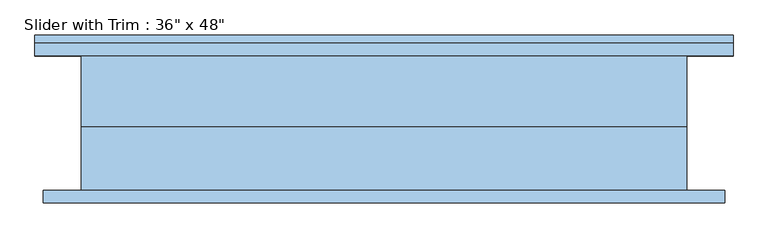
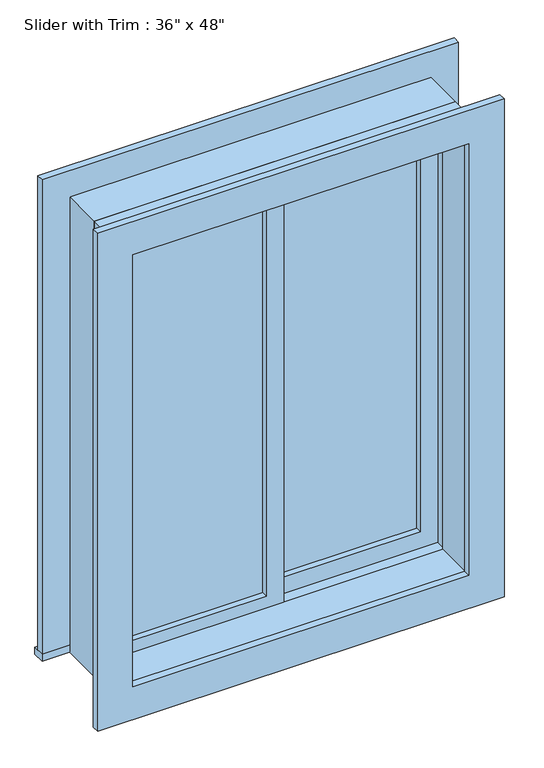
"""IFC4 building model written with IfcOpenShell, lengths in millimetres: window geometry."""

from ifc_helpers import new_model, si_unit, frame, origin, place, context, project, spatial, polyline, outline, extrude, source, transform, mapped, element, save


def window_54100e87(model_context):
    return source(origin(), model_context, "Body", "SweptSolid", [
        extrude(outline(polyline([(-393.7, 22.225), (-22.225, 22.225), (-22.225, 9.525), (-393.7, 9.525), (-393.7, 22.225)])), frame((0.0, 0.0, 977.9), z_axis=(0.0, 0.0, 1.0), x_axis=(1.0, 0.0, 0.0)), (0.0, 0.0, 1.0), 1092.2),
        extrude(outline(polyline([(2114.55, -438.15), (933.45, -438.15), (933.45, 22.225), (2114.55, 22.225), (2114.55, -438.15)]), holes=[polyline([(2070.1, -393.7), (2070.1, -22.225), (977.9, -22.225), (977.9, -393.7), (2070.1, -393.7)])]), frame((0.0, -6.35, 0.0), z_axis=(0.0, 1.0, 0.0), x_axis=(0.0, 0.0, 1.0)), (0.0, 0.0, 1.0), 44.45),
        extrude(outline(polyline([(-527.05, 133.35), (527.05, 133.35), (527.05, 101.6), (-527.05, 101.6), (-527.05, 133.35)])), frame((0.0, 0.0, 914.4), z_axis=(0.0, 0.0, 1.0), x_axis=(1.0, 0.0, 0.0)), (0.0, 0.0, 1.0), 19.05),
        extrude(outline(polyline([(2114.55, -438.15), (2114.55, 438.15), (933.45, 438.15), (933.45, 527.05), (2203.45, 527.05), (2203.45, -527.05), (933.45, -527.05), (933.45, -438.15), (2114.55, -438.15)])), frame((0.0, 101.6, 0.0), z_axis=(0.0, 1.0, 0.0), x_axis=(0.0, 0.0, 1.0)), (0.0, 0.0, 1.0), 19.05),
        extrude(outline(polyline([(2190.75, 514.35), (2190.75, -514.35), (857.25, -514.35), (857.25, 514.35), (2190.75, 514.35)]), holes=[polyline([(2101.85, 425.45), (946.15, 425.45), (946.15, -425.45), (2101.85, -425.45), (2101.85, 425.45)])]), frame((0.0, -120.65, 0.0), z_axis=(0.0, 1.0, 0.0), x_axis=(0.0, 0.0, 1.0)), (0.0, 0.0, 1.0), 19.05),
        extrude(outline(polyline([(393.7, 53.975), (22.225, 53.975), (22.225, 66.675), (393.7, 66.675), (393.7, 53.975)])), frame((0.0, 0.0, 977.9), z_axis=(0.0, 0.0, 1.0), x_axis=(1.0, 0.0, 0.0)), (0.0, 0.0, 1.0), 1092.2),
        extrude(outline(polyline([(2114.55, -22.225), (933.45, -22.225), (933.45, 438.15), (2114.55, 438.15), (2114.55, -22.225)]), holes=[polyline([(2070.1, 22.225), (2070.1, 393.7), (977.9, 393.7), (977.9, 22.225), (2070.1, 22.225)])]), frame((0.0, 38.1, 0.0), z_axis=(0.0, 1.0, 0.0), x_axis=(0.0, 0.0, 1.0)), (0.0, 0.0, 1.0), 44.45),
        extrude(outline(polyline([(2133.6, -457.2), (914.4, -457.2), (914.4, 457.2), (2133.6, 457.2), (2133.6, -457.2)]), holes=[polyline([(2101.85, -425.45), (2101.85, 425.45), (946.15, 425.45), (946.15, -425.45), (2101.85, -425.45)])]), frame((0.0, -101.6, 0.0), z_axis=(0.0, 1.0, 0.0), x_axis=(0.0, 0.0, 1.0)), (0.0, 0.0, 1.0), 95.25),
        extrude(outline(polyline([(2133.6, 457.2), (2133.6, -457.2), (914.4, -457.2), (914.4, 457.2), (2133.6, 457.2)]), holes=[polyline([(2114.55, 438.15), (933.45, 438.15), (933.45, -438.15), (2114.55, -438.15), (2114.55, 438.15)])]), frame((0.0, -6.35, 0.0), z_axis=(0.0, 1.0, 0.0), x_axis=(0.0, 0.0, 1.0)), (0.0, 0.0, 1.0), 107.95),
    ])


if __name__ == "__main__":
    model = new_model("IFC4")
    model_context = context("Model", 3, world=origin())
    ifc_project = project(units=[si_unit("LENGTHUNIT", "METRE", prefix="MILLI")], contexts=[model_context])
    site = spatial("IfcSite", under=ifc_project)
    building = spatial("IfcBuilding", under=site)
    placement = place(None, origin())
    window_shape = window_54100e87(model_context)
    element("IfcWindow", 1, ObjectType="Slider with Trim : 36\" x 48\"", at=placement, inside=building, context=model_context, shape_type="MappedRepresentation", body=[
        mapped(window_shape, transform((0.0, 0.0, 0.0), x_axis=(1.0, 0.0, 0.0), y_axis=(0.0, 1.0, 0.0), z_axis=(0.0, 0.0, 1.0))),
    ])
    save(model, "model.ifc")

# Revit data of these elements
# Type "Slider with Trim : 36\" x 48\""
#   Type Mark = "22"
#   Construction Type Id = "GSP4R"
#   Assembly Code = "B2020100"
#   Analytic Construction = "1/8 in Pilkington single glazing"
#   Visual Light Transmittance = 0.9
#   Solar Heat Gain Coefficient = 0.78
#   Heat Transfer Coefficient (U) = 0.6496 BTU/(h·ft²·°F)
#   Height = 4' - 0"
#   Default Sill Height = 3' - 0"
#   Trim Projection - Ext. = 0' - 0 3/4"
#   Trim Projection - Int. = 0' - 0 3/4"
#   Trim Width - Exterior = 0' - 3 1/2"
#   Trim Width - Interior = 0' - 3 1/2"
#   Width = 3' - 0"
#   Window Inset = 0' - 0 3/4"
#   Define Thermal Properties by = 1
#   Glass Pane Material = Glass
#   Sash Material = Sash
#   Trim Exterior Material = Trim
#   Trim Interior Material = Trim
#   Wall Closure = (empty or 0)
# Element 1 (IfcWindow, "Slider with Trim : 36\" x 48\"")
#   Materials on its faces: "Sash", "Trim", "Glass"
# Materials
#   "Glass": class "Glass", colour RGB 0 128 192, transparency 0.75, Description = "Soda Lime Glass", Cost = 0
#   "Sash": class "Wood", colour RGB 224 178 126, transparency 0
#   "Trim": class "Wood", colour RGB 224 178 126, transparency 0
